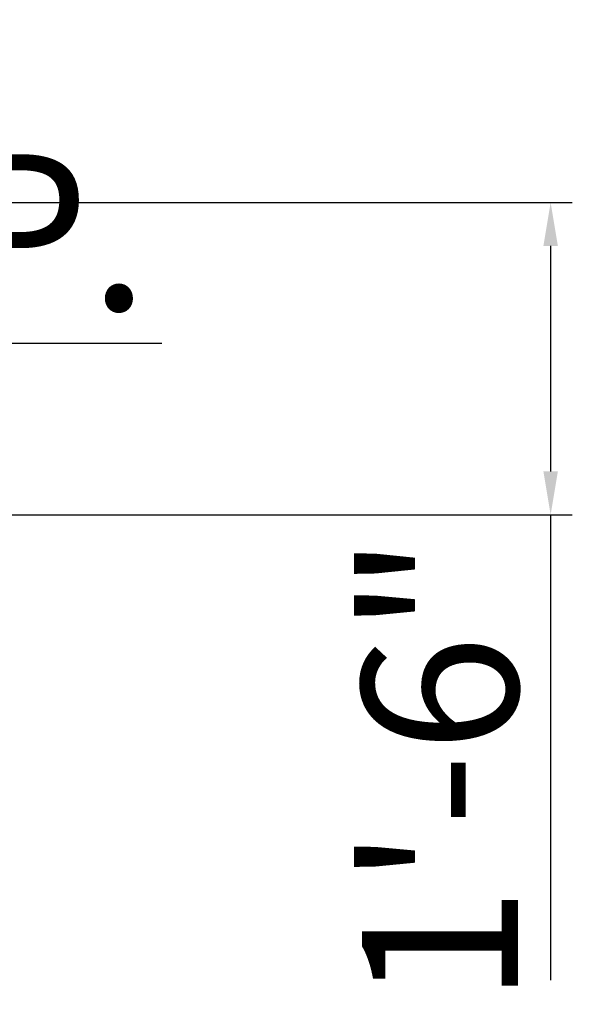
# Model space of a CAD drawing. Units: inches. Extents: x 2337 to 3570, y 1258 to 1938.
# Tile 28 of 30: x 3471 to 3502, y 1496 to 1553. Entities that reach past the tile are written whole.
import ezdxf

# ---------------------------------------------------------------- set-up
doc = ezdxf.new("R2010")
doc.units = ezdxf.units.IN
doc.layers.add('A-ANNO-DIMS', color=2, linetype='Continuous', lineweight=18)
doc.styles.get("Standard").update_dxf_attribs({"font": 'arial.ttf'})
doc.dimstyles.new('ISO-25', dxfattribs={"dimtxt": 9, "dimasz": 2.5, "dimexe": 1.25, "dimexo": 0.625, "dimtad": 1, "dimdec": 1, "dimlunit": 3, "dimtxsty": 'Standard', "dimcen": 2.5, "dimadec": 0, "dimazin": 0, "dimtfac": 1, "dimtdec": 1, "dimtmove": 0, "dimatfit": 3, "dimfxl": 1, "dimarcsym": 0})

# ---------------------------------------------------------------- blocks, each defined once
blk = doc.blocks.new('*D69')
at = {"layer": 'A-ANNO-DIMS', "color": 0, "lineweight": -2, "transparency": 16777216}
for p, q in [((3371.786, 1541.491), (3371.786, 1532.766)), ((3419.786, 1541.491), (3419.786, 1532.766)), ((3374.286, 1534.016), (3417.286, 1534.016)), ((3419.786, 1534.016), (3478.758, 1534.016))]:
    blk.add_line(p, q, dxfattribs=at)
at = {"layer": 'A-ANNO-DIMS', "color": 0, "transparency": 16777216}
for points in [[(3374.286, 1534.433), (3374.286, 1533.599), (3371.786, 1534.016)], [(3417.286, 1534.433), (3417.286, 1533.599), (3419.786, 1534.016)]]:
    blk.add_solid(points, dxfattribs=at)
at = {"layer": 'Defpoints', "color": 0, "transparency": 16777216}
for p in [(3371.786, 1542.116), (3419.786, 1542.116), (3419.786, 1534.016)]:
    blk.add_point(p, dxfattribs=at)
at = {"layer": 'A-ANNO-DIMS', "color": 0, "transparency": 16777216, "insert": (3450.522, 1539.236), "char_height": 9, "attachment_point": 5}
blk.add_mtext('4\'-0" TYP.', dxfattribs=at)
blk = doc.blocks.new('*D115')
at = {"layer": 'A-ANNO-DIMS', "color": 0, "lineweight": -2, "transparency": 16777216}
for p, q in [((3243.411, 1542.116), (3502.436, 1542.116)), ((3501.186, 1539.616), (3501.186, 1526.616)), ((3243.411, 1524.116), (3502.436, 1524.116)), ((3501.186, 1524.116), (3501.186, 1497.289))]:
    blk.add_line(p, q, dxfattribs=at)
at = {"layer": 'A-ANNO-DIMS', "color": 0, "transparency": 16777216}
for points in [[(3500.769, 1539.616), (3501.603, 1539.616), (3501.186, 1542.116)], [(3500.769, 1526.616), (3501.603, 1526.616), (3501.186, 1524.116)]]:
    blk.add_solid(points, dxfattribs=at)
at = {"layer": 'Defpoints', "color": 0, "transparency": 16777216}
for p in [(3242.786, 1542.116), (3242.786, 1524.116), (3501.186, 1524.116)]:
    blk.add_point(p, dxfattribs=at)
at = {"layer": 'A-ANNO-DIMS', "color": 0, "transparency": 16777216, "insert": (3495.966, 1509.452), "char_height": 9, "attachment_point": 5, "rotation": 90}
blk.add_mtext('1\'-6"', dxfattribs=at)

msp = doc.modelspace()

# ---------------------------------------------------------------- dimensions: what is measured, and where the dimension line sits
at = {"layer": 'A-ANNO-DIMS'}
dim = msp.add_linear_dim(base=(3419.786, 1534.016), p1=(3371.786, 1542.116), p2=(3419.786, 1542.116), text='<> TYP.', dimstyle='ISO-25', override={"dimdec": 1, "dimlfac": 1, "dimrnd": 0, "dimzin": 1, "dimdsep": 46, "dimlunit": 4, "dimfrac": 2}, dxfattribs=at)
dim.commit()
dim.dimension.update_dxf_attribs({"geometry": '*D69', "text_midpoint": (3450.522, 1539.236)})
dim = msp.add_linear_dim(base=(3501.186, 1524.116), p1=(3242.786, 1542.116), p2=(3242.786, 1524.116), angle=90, dimstyle='ISO-25', override={"dimdec": 1, "dimlfac": 1, "dimrnd": 0, "dimzin": 1, "dimdsep": 46, "dimlunit": 4, "dimfrac": 2}, dxfattribs=at)
dim.commit()
dim.dimension.update_dxf_attribs({"geometry": '*D115', "text_midpoint": (3495.966, 1509.452)})

doc.saveas('drawing.dxf')
